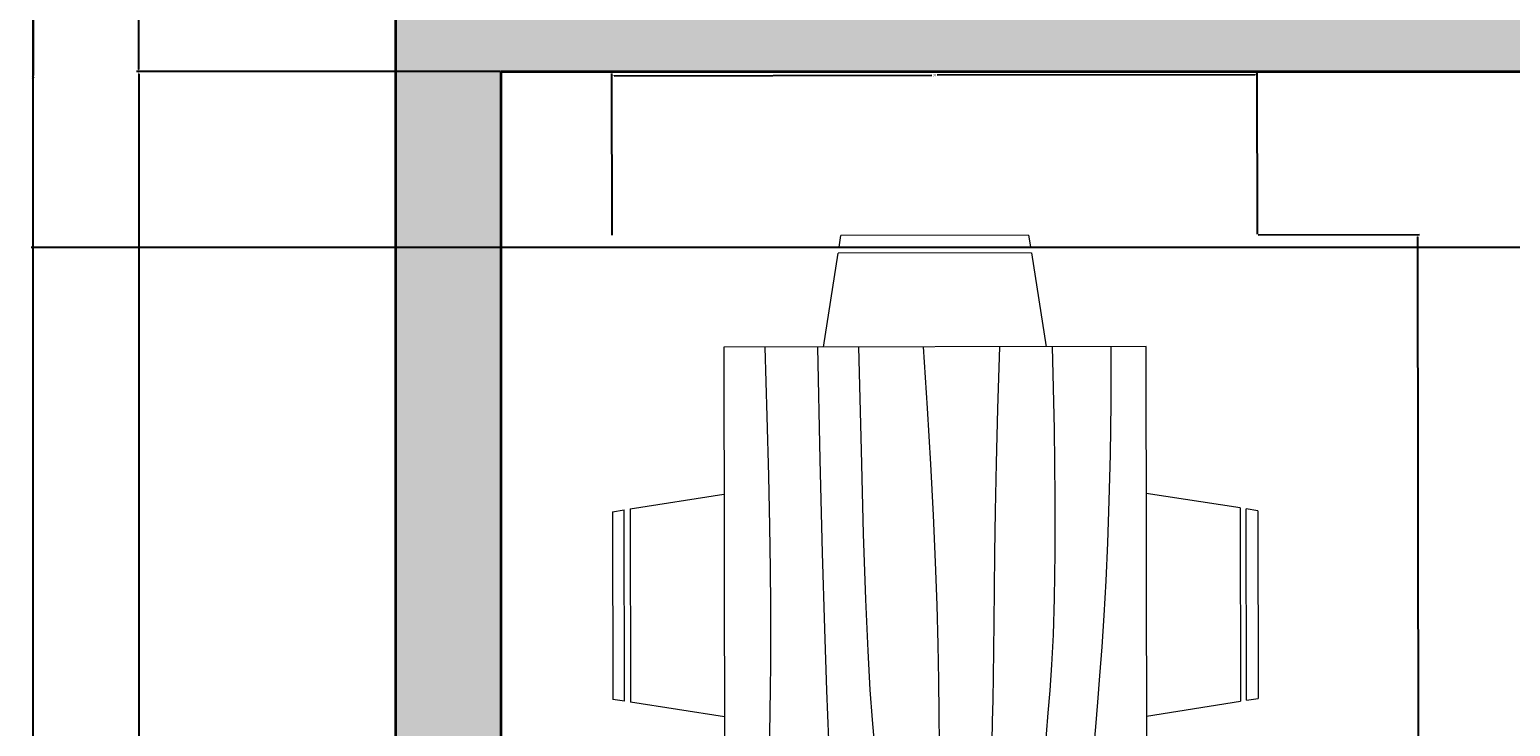
# Model space of a CAD drawing. Units: inches. Extents: x -30 to 437, y -29 to 647.
# Tile 2 of 15: x -30 to 97, y 113 to 172. Entities that reach past the tile are written whole.
import ezdxf

# ---------------------------------------------------------------- set-up
doc = ezdxf.new("R2010")
doc.units = ezdxf.units.IN
doc.header["$MEASUREMENT"] = 0
for name, color, linetype, lineweight in [('A-ANNO-DIMS', 2, 'Continuous', 18), ('A-WALL', 7, 'Continuous', 35), ('furniture', 220, 'Continuous', 18)]:
    doc.layers.add(name, color=color, linetype=linetype, lineweight=lineweight)
doc.layers.add('A-WALL-PATT', color=251, linetype='Continuous', lineweight=13, true_color=0x636466)
doc.styles.get("Standard").update_dxf_attribs({"font": 'arial.ttf'})
doc.dimstyles.get("Standard").update_dxf_attribs({"dimtxt": 0.18, "dimasz": 0.18, "dimexe": 0.18, "dimexo": 0.0625, "dimgap": 0.09, "dimtad": 0, "dimtih": 1, "dimtoh": 1, "dimdec": 4, "dimzin": 0, "dimdsep": 46, "dimtxsty": 'Standard', "dimcen": 0.09, "dimadec": 0, "dimazin": 0, "dimtfac": 1, "dimtdec": 4, "dimtofl": 0, "dimtmove": 0, "dimatfit": 3, "dimfxl": 1, "dimtolj": 1, "dimtzin": 0, "dimarcsym": 0})

# ---------------------------------------------------------------- blocks, each defined once
blk = doc.blocks.new('Dining Set - 36 x 72 in.')
for p, q in [((-22, 27.5), (-22.1562, 26.50042)), ((-22, 27.5), (-6, 27.5)), ((-5.8437, 26.49966), (-6, 27.5)), ((6, 27.5), (5.8438, 26.50042)), ((6, 27.5), (22, 27.5)), ((22.1563, 26.49966), (22, 27.5)), ((-22.2343, 26.00059), (-23.4847, 17.99762)), ((-22.2304, 26), (-5.7608, 26)), ((-5.8416, 26.5), (-22.1534, 26.5)), ((-4.5152, 17.99762), (-5.7655, 25.99926)), ((5.7657, 26.00059), (4.5153, 17.99762)), ((5.7696, 26), (22.2392, 26)), ((22.1584, 26.5), (5.8466, 26.5)), ((23.4848, 17.99762), (22.2345, 25.99926)), ((36, 18), (-36, 18)), ((-36, 18), (-36, -18)), ((36, -18), (36, 18)), ((-44.0006, 8.23428), (-35.9976, 9.48474)), ((44.0006, 8.23428), (35.9976, 9.48474)), ((-45.5, 8), (-44.5004, 8.15617)), ((-45.5, 8), (-45.5, -8)), ((-44.5, -8.15843), (-44.5, 8.15338)), ((-44, 8.23041), (-44, -8.23915)), ((44, 8.23041), (44, -8.23915)), ((44.5, -8.15843), (44.5, 8.15338)), ((45.5, 8), (44.5005, 8.15617)), ((45.5, 8), (45.5, -8)), ((-44.4997, -8.15631), (-45.5, -8)), ((-35.9976, -9.48476), (-43.9993, -8.2345)), ((35.9976, -9.48476), (43.9993, -8.2345)), ((44.4997, -8.15631), (45.5, -8)), ((-36, -18), (36, -18)), ((-22.2343, -26.0006), (-23.4847, -17.99762)), ((-4.5152, -17.99762), (-5.7655, -25.99928)), ((5.7657, -26.0006), (4.5153, -17.99762)), ((23.4848, -17.99762), (22.2345, -25.99928)), ((-22.2304, -26), (-5.7608, -26)), ((-22, -27.5), (-22.1562, -26.50044)), ((-5.8416, -26.5), (-22.1534, -26.5)), ((-5.8437, -26.49967), (-6, -27.5)), ((5.7696, -26), (22.2392, -26)), ((6, -27.5), (5.8438, -26.50044)), ((22.1584, -26.5), (5.8466, -26.5)), ((22.1563, -26.49967), (22, -27.5)), ((-22, -27.5), (-6, -27.5)), ((6, -27.5), (22, -27.5))]:
    blk.add_line(p, q)
for points in [[(-36, 15), (-31.1772, 14.97754), (-26.8079, 14.91406), (-22.8538, 14.81543), (-19.276, 14.6875), (-16.0362, 14.53613), (-13.0957, 14.36718), (-10.4159, 14.18652), (-7.9583, 14), (-5.6904, 13.81315), (-3.6035, 13.63021), (-1.6954, 13.45508), (0.0365, 13.29166), (1.5945, 13.14388), (2.9811, 13.01562), (4.1988, 12.9108), (5.25, 12.83333), (6.1393, 12.78613), (6.8802, 12.76823), (7.4883, 12.77767), (7.9792, 12.8125), (8.3685, 12.87077), (8.6719, 12.95052), (8.9049, 13.0498), (9.0833, 13.16666), (9.2205, 13.29899), (9.3216, 13.44401), (9.3895, 13.59879), (9.4271, 13.76041), (9.4373, 13.92594), (9.4232, 14.09245), (9.3875, 14.257), (9.3333, 14.41666), (9.2638, 14.56917), (9.1836, 14.71484), (9.0975, 14.85465), (9.0104, 14.98958), (8.9272, 15.1206), (8.8529, 15.2487), (8.7922, 15.37483), (8.75, 15.5), (8.7305, 15.62467), (8.7344, 15.74739), (8.7617, 15.86621), (8.8125, 15.97916), (8.8867, 16.08431), (8.9844, 16.17968), (9.1055, 16.26334), (9.25, 16.33333), (9.4189, 16.38802), (9.6172, 16.42708), (9.8506, 16.45052), (10.125, 16.45833), (10.4463, 16.45052), (10.8203, 16.42708), (11.2529, 16.38802), (11.75, 16.33333), (12.3184, 16.26318), (12.9694, 16.17838), (13.7151, 16.07991), (14.5677, 15.96875), (15.5395, 15.84586), (16.6426, 15.71224), (17.8893, 15.56884), (19.2917, 15.41666), (20.859, 15.25667), (22.5879, 15.08984), (24.4721, 14.91715), (26.5052, 14.73958), (28.6809, 14.5581), (30.9929, 14.3737), (33.4347, 14.18733), (36, 14)], [(-36, 10), (-28.9766, 10.14274), (-23.1725, 10.20442), (-18.4241, 10.19775), (-14.5677, 10.13541), (-11.4399, 10.03011), (-8.877, 9.89453), (-6.7154, 9.74137), (-4.7917, 9.58333), (-2.9698, 9.43082), (-1.2246, 9.28515), (0.4415, 9.14534), (2.026, 9.01041), (3.5266, 8.87939), (4.9408, 8.7513), (6.266, 8.62516), (7.5, 8.5), (8.6411, 8.37549), (9.6914, 8.2539), (10.6538, 8.13818), (11.5312, 8.03125), (12.3267, 7.93603), (13.043, 7.85547), (13.6831, 7.79248), (14.25, 7.75), (14.7471, 7.7303), (15.1797, 7.73307), (15.5537, 7.75732), (15.875, 7.80208), (16.1494, 7.86637), (16.3828, 7.94922), (16.5811, 8.04964), (16.75, 8.16666), (16.8944, 8.29915), (17.0143, 8.44531), (17.1089, 8.60319), (17.1771, 8.77083), (17.218, 8.94629), (17.2305, 9.1276), (17.2137, 9.31282), (17.1667, 9.5), (17.0895, 9.6875), (16.987, 9.875), (16.8649, 10.0625), (16.7292, 10.25), (16.5856, 10.4375), (16.4401, 10.625), (16.2985, 10.8125), (16.1667, 11), (16.05, 11.18733), (15.9518, 11.3737), (15.8752, 11.5581), (15.8229, 11.73958), (15.798, 11.91715), (15.8034, 12.08984), (15.842, 12.25667), (15.9167, 12.41666), (16.0295, 12.56836), (16.1784, 12.70833), (16.3605, 12.83268), (16.5729, 12.9375), (16.8127, 13.01888), (17.0768, 13.07291), (17.3625, 13.0957), (17.6667, 13.08333), (17.9894, 13.03312), (18.3418, 12.94726), (18.7382, 12.82918), (19.1927, 12.68229), (19.7195, 12.51001), (20.3327, 12.31575), (21.0465, 12.10294), (21.875, 11.875), (22.8357, 11.63354), (23.959, 11.37304), (25.2786, 11.08618), (26.8282, 10.76562), (28.6414, 10.40405), (30.752, 9.99414), (33.1936, 9.52856), (36, 9)], [(-36, 5.5), (-30.7157, 5.3348), (-26.069, 5.20963), (-21.9946, 5.11767), (-18.4271, 5.05208), (-15.3009, 5.00602), (-12.5508, 4.97265), (-10.1112, 4.94515), (-7.9167, 4.91666), (-5.909, 4.88167), (-4.0586, 4.83984), (-2.3429, 4.79215), (-0.7396, 4.73958), (0.7739, 4.6831), (2.22, 4.6237), (3.6213, 4.56233), (5, 4.5), (6.373, 4.43782), (7.7344, 4.3776), (9.0723, 4.32129), (10.375, 4.27083), (11.6309, 4.22819), (12.8281, 4.19531), (13.9551, 4.17415), (15, 4.16666), (15.954, 4.17448), (16.819, 4.19791), (17.6001, 4.23698), (18.3021, 4.29166), (18.9299, 4.36198), (19.4883, 4.44791), (19.9823, 4.54948), (20.4167, 4.66666), (20.7969, 4.79899), (21.1302, 4.94401), (21.4245, 5.09879), (21.6875, 5.26041), (21.9271, 5.42594), (22.1511, 5.59245), (22.3672, 5.757), (22.5834, 5.91666), (22.8065, 6.06868), (23.0404, 6.21093), (23.2879, 6.34147), (23.5521, 6.45833), (23.8358, 6.55957), (24.142, 6.64323), (24.4735, 6.70735), (24.8334, 6.75), (25.2235, 6.76969), (25.642, 6.76692), (26.0858, 6.74267), (26.5521, 6.69791), (27.0379, 6.63362), (27.5404, 6.55078), (28.0565, 6.45036), (28.5834, 6.33333), (29.1242, 6.19987), (29.7071, 6.04687), (30.3661, 5.87044), (31.1354, 5.66666), (32.0493, 5.43164), (33.142, 5.16146), (34.4475, 4.85221), (36, 4.5)], [(-36, -1), (-30.7915, -0.6591), (-26.0195, -0.38216), (-21.6519, -0.16284), (-17.6563, 0.00521), (-14.0005, 0.12833), (-10.6523, 0.21289), (-7.5796, 0.26522), (-4.75, 0.29166), (-2.134, 0.29793), (0.2878, 0.28711), (2.5317, 0.26163), (4.6146, 0.22396), (6.5529, 0.17651), (8.3633, 0.12174), (10.0623, 0.06209), (11.6667, 0), (13.1899, -0.06201), (14.6341, -0.1211), (15.9982, -0.17432), (17.2813, -0.21875), (18.4823, -0.25147), (19.6003, -0.26953), (20.6343, -0.27002), (21.5834, -0.25), (22.4481, -0.20768), (23.2357, -0.14584), (23.9549, -0.06836), (24.6146, 0.02083), (25.2235, 0.11784), (25.7904, 0.21875), (26.3241, 0.31966), (26.8334, 0.41666), (27.3265, 0.50618), (27.8099, 0.58593), (28.2894, 0.65397), (28.7709, 0.70833), (29.2601, 0.74707), (29.763, 0.76823), (30.2855, 0.76985), (30.8334, 0.75), (31.4088, 0.70784), (31.9994, 0.64713), (32.589, 0.57275), (33.1615, 0.48958), (33.7008, 0.4025), (34.1908, 0.3164), (34.6153, 0.23616), (34.9584, 0.16666), (35.2099, 0.11165), (35.3848, 0.07031), (35.504, 0.04069), (35.5886, 0.02083), (35.6594, 0.00879), (35.7377, 0.0026), (35.8442, 0.00032), (36, 0)], [(-36, -6.5), (-27.1843, -6.31267), (-20.084, -6.1263), (-14.469, -5.9419), (-10.1094, -5.76042), (-6.7752, -5.58285), (-4.2363, -5.41016), (-2.2629, -5.24333), (-0.625, -5.08334), (0.8708, -4.93099), (2.2715, -4.78646), (3.5872, -4.64974), (4.8281, -4.52084), (6.0046, -4.39974), (7.127, -4.28646), (8.2053, -4.18099), (9.25, -4.08334), (10.2705, -3.99382), (11.2734, -3.91407), (12.2647, -3.84603), (13.25, -3.79167), (14.2354, -3.75293), (15.2266, -3.73177), (16.2295, -3.73015), (17.25, -3.75), (18.2912, -3.79248), (19.3451, -3.85547), (20.4009, -3.93604), (21.4479, -4.03125), (22.4754, -4.13819), (23.4727, -4.25391), (24.4289, -4.37549), (25.3334, -4.5), (26.1785, -4.62492), (26.9694, -4.74935), (27.7145, -4.87281), (28.4219, -4.99479), (29.1, -5.11483), (29.7572, -5.23242), (30.4016, -5.34709), (31.0417, -5.45834), (31.6837, -5.56437), (32.3262, -5.65821), (32.9658, -5.73153), (33.599, -5.77604), (34.2224, -5.78345), (34.8327, -5.74545), (35.4264, -5.65373), (36, -5.5)], [(-36, -10), (-26.4022, -9.81299), (-18.4675, -9.62891), (-11.9839, -9.45069), (-6.7396, -9.28125), (-2.5226, -9.12354), (0.8789, -8.98047), (3.6769, -8.85498), (6.0833, -8.75), (8.2767, -8.66765), (10.3021, -8.60677), (12.1712, -8.56543), (13.8958, -8.54167), (15.4876, -8.53353), (16.9583, -8.53907), (18.3197, -8.55632), (19.5834, -8.58334), (20.7616, -8.61841), (21.8685, -8.66081), (22.9188, -8.71004), (23.9271, -8.76563), (24.9081, -8.82707), (25.8763, -8.89388), (26.8465, -8.96558), (27.8334, -9.04167), (28.8474, -9.12118), (29.8828, -9.20117), (30.93, -9.27824), (31.9792, -9.34896), (33.0205, -9.40991), (34.0443, -9.45768), (35.0407, -9.48885), (36, -9.5)], [(-36, -14.5), (-30.0881, -14.33513), (-25.0332, -14.21224), (-20.7312, -14.12647), (-17.0781, -14.07292), (-13.97, -14.04671), (-11.3027, -14.04297), (-8.9724, -14.05681), (-6.875, -14.08334), (-4.9224, -14.11833), (-3.0905, -14.16016), (-1.3709, -14.20785), (0.2448, -14.26042), (1.7647, -14.3169), (3.1973, -14.3763), (4.5507, -14.43767), (5.8333, -14.5), (7.0554, -14.5621), (8.235, -14.62175), (9.3922, -14.67652), (10.5469, -14.72396), (11.7192, -14.76164), (12.929, -14.78711), (14.1965, -14.79794), (15.5417, -14.79167), (16.9933, -14.76424), (18.6152, -14.70508), (20.4804, -14.60197), (22.6615, -14.44271), (25.2312, -14.21509), (28.2624, -13.9069), (31.8277, -13.50594), (36, -13)]]:
    blk.add_lwpolyline(points)
blk = doc.blocks.new('*D19')
at = {"layer": 'A-ANNO-DIMS', "color": 0, "lineweight": -2, "transparency": 16777216}
for p, q in [((75.18, 154.64), (88.95, 154.66)), ((88.77, 154.48), (88.84, 109.34)), ((88.91, 63.84), (88.84, 108.98)), ((75.32, 63.64), (89.09, 63.66))]:
    blk.add_line(p, q, dxfattribs=at)
at = {"layer": 'A-ANNO-DIMS', "color": 0, "transparency": 16777216}
for points in [[(88.8, 154.48), (88.74, 154.48), (88.77, 154.66)], [(88.94, 63.84), (88.88, 63.84), (88.91, 63.66)]]:
    blk.add_solid(points, dxfattribs=at)
at = {"layer": 'Defpoints', "color": 0, "transparency": 16777216}
for p in [(75.12, 154.64), (75.26, 63.64), (88.91, 63.66)]:
    blk.add_point(p, dxfattribs=at)
at = {"layer": 'A-ANNO-DIMS', "color": 0, "transparency": 16777216, "insert": (88.84, 109.16), "char_height": 0.18, "attachment_point": 5}
blk.add_mtext('\\A1;DINING SET 91', dxfattribs=at)
blk = doc.blocks.new('*D20')
at = {"layer": 'A-ANNO-DIMS', "color": 0, "lineweight": -2, "transparency": 16777216}
for p, q in [((20.12, 154.62), (20.1, 168.38)), ((20.28, 168.2), (47.38, 168.25)), ((74.92, 168.29), (47.82, 168.25)), ((75.12, 154.7), (75.1, 168.47))]:
    blk.add_line(p, q, dxfattribs=at)
at = {"layer": 'A-ANNO-DIMS', "color": 0, "transparency": 16777216}
for points in [[(20.28, 168.23), (20.28, 168.17), (20.1, 168.2)], [(74.92, 168.32), (74.92, 168.26), (75.1, 168.29)]]:
    blk.add_solid(points, dxfattribs=at)
at = {"layer": 'Defpoints', "color": 0, "transparency": 16777216}
for p in [(75.1, 168.29), (20.12, 154.55), (75.12, 154.64)]:
    blk.add_point(p, dxfattribs=at)
at = {"layer": 'A-ANNO-DIMS', "color": 0, "transparency": 16777216, "insert": (47.6, 168.25), "char_height": 0.18, "attachment_point": 5}
blk.add_mtext('\\A1;55', dxfattribs=at)
blk = doc.blocks.new('*D26')
at = {"layer": 'A-ANNO-DIMS', "color": 0, "lineweight": -2, "transparency": 16777216}
for p, q in [((1.61, 615.55), (-29.41, 615.55)), ((-29.23, 615.37), (-29.23, 308.98)), ((-29.23, 2.23), (-29.23, 308.62)), ((1.61, 2.05), (-29.41, 2.05))]:
    blk.add_line(p, q, dxfattribs=at)
at = {"layer": 'A-ANNO-DIMS', "color": 0, "transparency": 16777216}
for points in [[(-29.26, 615.37), (-29.2, 615.37), (-29.23, 615.55)], [(-29.26, 2.23), (-29.2, 2.23), (-29.23, 2.05)]]:
    blk.add_solid(points, dxfattribs=at)
at = {"layer": 'Defpoints', "color": 0, "transparency": 16777216}
for p in [(-29.23, 615.55), (1.67, 615.55), (1.67, 2.05)]:
    blk.add_point(p, dxfattribs=at)
at = {"layer": 'A-ANNO-DIMS', "color": 0, "transparency": 16777216, "insert": (-29.23, 308.8), "char_height": 0.18, "attachment_point": 5}
blk.add_mtext('\\A1;613.5', dxfattribs=at)
blk = doc.blocks.new('*D30')
at = {"layer": 'A-ANNO-DIMS', "color": 0, "lineweight": -2, "transparency": 16777216}
for p, q in [((10.61, 168.55), (-20.41, 168.55)), ((-20.23, 168.37), (-20.23, 89.98)), ((-20.23, 11.23), (-20.23, 89.62)), ((10.61, 11.05), (-20.41, 11.05))]:
    blk.add_line(p, q, dxfattribs=at)
at = {"layer": 'A-ANNO-DIMS', "color": 0, "transparency": 16777216}
for points in [[(-20.26, 168.37), (-20.2, 168.37), (-20.23, 168.55)], [(-20.26, 11.23), (-20.2, 11.23), (-20.23, 11.05)]]:
    blk.add_solid(points, dxfattribs=at)
at = {"layer": 'Defpoints', "color": 0, "transparency": 16777216}
for p in [(-20.23, 168.55), (10.67, 168.55), (10.67, 11.05)]:
    blk.add_point(p, dxfattribs=at)
at = {"layer": 'A-ANNO-DIMS', "color": 0, "transparency": 16777216, "insert": (-20.23, 89.8), "char_height": 0.18, "attachment_point": 5}
blk.add_mtext('\\A1;157.5', dxfattribs=at)
blk = doc.blocks.new('*D31')
at = {"layer": 'A-ANNO-DIMS', "color": 0, "lineweight": -2, "transparency": 16777216}
for p, q in [((10.61, 233.55), (-20.41, 233.55)), ((-20.23, 233.37), (-20.23, 201.23)), ((-20.23, 168.73), (-20.23, 200.87)), ((10.61, 168.55), (-20.41, 168.55))]:
    blk.add_line(p, q, dxfattribs=at)
at = {"layer": 'A-ANNO-DIMS', "color": 0, "transparency": 16777216}
for points in [[(-20.26, 233.37), (-20.2, 233.37), (-20.23, 233.55)], [(-20.26, 168.73), (-20.2, 168.73), (-20.23, 168.55)]]:
    blk.add_solid(points, dxfattribs=at)
at = {"layer": 'Defpoints', "color": 0, "transparency": 16777216}
for p in [(-20.23, 233.55), (10.67, 233.55), (10.67, 168.55)]:
    blk.add_point(p, dxfattribs=at)
at = {"layer": 'A-ANNO-DIMS', "color": 0, "transparency": 16777216, "insert": (-20.23, 201.05), "char_height": 0.18, "attachment_point": 5}
blk.add_mtext('\\A1;65', dxfattribs=at)
blk = doc.blocks.new('*D52')
at = {"layer": 'A-ANNO-DIMS', "color": 0, "lineweight": -2, "transparency": 16777216}
for p, q in [((367.61, 182.55), (-29.41, 182.55)), ((-29.23, 182.37), (-29.23, 168.23)), ((-29.23, 153.73), (-29.23, 167.87)), ((396.61, 153.55), (-29.41, 153.55))]:
    blk.add_line(p, q, dxfattribs=at)
at = {"layer": 'A-ANNO-DIMS', "color": 0, "transparency": 16777216}
for points in [[(-29.26, 182.37), (-29.2, 182.37), (-29.23, 182.55)], [(-29.26, 153.73), (-29.2, 153.73), (-29.23, 153.55)]]:
    blk.add_solid(points, dxfattribs=at)
at = {"layer": 'Defpoints', "color": 0, "transparency": 16777216}
for p in [(367.67, 182.55), (-29.23, 153.55), (396.67, 153.55)]:
    blk.add_point(p, dxfattribs=at)
at = {"layer": 'A-ANNO-DIMS', "color": 0, "transparency": 16777216, "insert": (-29.23, 168.05), "char_height": 0.18, "attachment_point": 5}
blk.add_mtext('\\A1;29', dxfattribs=at)

msp = doc.modelspace()

# ---------------------------------------------------------------- hatches: boundary and pattern name
at = {"layer": 'A-WALL-PATT'}
h = msp.add_hatch(color=256, dxfattribs=at)
h.dxf.hatch_style = 1
h.paths.add_polyline_path([(393.6054, 183.2352), (369.6054, 183.2352), (369.6054, 213.2352), (393.6054, 213.2352), (393.6054, 207.2352), (394.6054, 207.2352), (394.6054, 211.2352), (395.6054, 211.2352), (395.6054, 185.2352), (394.6054, 185.2352), (394.6054, 189.2352), (393.6054, 189.2352)], flags=0)
h.paths.add_polyline_path([(384.6054, 189.2352, -1), (390.6054, 189.2352, -1)], flags=0)
h.paths.add_polyline_path([(385.6054, 189.2352, -1), (389.6054, 189.2352, -1)], flags=0)
h.paths.add_polyline_path([(374.6054, 189.2352, -1), (382.6054, 189.2352, -1)], flags=0)
h.paths.add_polyline_path([(386.6054, 189.2352, -1), (388.6054, 189.2352, -1)], flags=0)
h.paths.add_polyline_path([(375.6054, 189.2352, -1), (381.6054, 189.2352, -1)], flags=0)
h.paths.add_polyline_path([(376.6054, 189.2352, -1), (380.6054, 189.2352, -1)], flags=0)
h.paths.add_polyline_path([(377.6054, 189.2352, -1), (379.6054, 189.2352, -1)], flags=0)
h.paths.add_polyline_path([(390.6054, 195.2352), (374.6054, 195.2352), (374.6054, 201.2352), (390.6054, 201.2352)], flags=0)
h.paths.add_polyline_path([(389.6054, 196.2352), (375.6054, 196.2352), (375.6054, 200.2352), (389.6054, 200.2352)], flags=0)
h.paths.add_polyline_path([(383.6054, 207.2352, -1), (391.6054, 207.2352, -1)], flags=0)
h.paths.add_polyline_path([(384.6054, 207.2352, -1), (390.6054, 207.2352, -1)], flags=0)
h.paths.add_polyline_path([(385.6054, 207.2352, -1), (389.6054, 207.2352, -1)], flags=0)
h.paths.add_polyline_path([(386.6054, 207.2352, -1), (388.6054, 207.2352, -1)], flags=0)
h.paths.add_polyline_path([(375.6054, 207.2352, -1), (381.6054, 207.2352, -1)], flags=0)
h.paths.add_polyline_path([(376.6054, 207.2352, -1), (380.6054, 207.2352, -1)], flags=0)
h.paths.add_polyline_path([(377.6054, 207.2352, -1), (379.6054, 207.2352, -1)], flags=0)
h.paths.add_polyline_path([(305.5437, 160.3663, -0.41421356), (304.0437, 158.8663), (271.0437, 158.8663, -0.41421356), (269.5437, 160.3663), (269.5437, 178.3663, -0.41421356), (271.0437, 179.8663), (304.0437, 179.8663, -0.41421356), (305.5437, 178.3663)], flags=0)
h.paths.add_polyline_path([(304.0437, 165.3663, -0.41421356), (303.0437, 164.3663), (289.2937, 164.3663, -0.41421356), (288.2937, 165.3663), (288.2937, 177.3663, -0.41421356), (289.2937, 178.3663), (303.0437, 178.3663, -0.41421356), (304.0437, 177.3663)], flags=0)
h.paths.add_polyline_path([(296.5437, 171.3663, -1), (295.5437, 171.3663, -1)], flags=0)
h.paths.add_polyline_path([(286.7937, 165.3663, -0.41421356), (285.7937, 164.3663), (272.0437, 164.3663, -0.41421356), (271.0437, 165.3663), (271.0437, 177.3663, -0.41421356), (272.0437, 178.3663), (285.7937, 178.3663, -0.41421356), (286.7937, 177.3663)], flags=0)
h.paths.add_polyline_path([(279.5437, 171.3663, -1), (278.5437, 171.3663, -1)], flags=0)
h.paths.add_polyline_path([(360.6737, 290.5474), (360.6737, 300.5474), (396.6737, 300.5474), (396.6737, 290.5474)], flags=0)
h.paths.add_polyline_path([(259.6737, 124.5474), (259.6737, 114.5474), (171.6737, 114.5474), (171.6737, 124.5474)], flags=0)
h.paths.add_polyline_path([(288.0737, 215.3705), (286.7097, 214.583), (268.7097, 245.7599), (270.0737, 246.5474)], flags=0)
h.paths.add_polyline_path([(259.6737, 168.5474), (256.6737, 168.5474), (256.6737, 173.5474), (256.6737, 179.0224), (255.8753, 177.6395), (224.2956, 195.872, 0.12053744), (220.1737, 179.0224, 0.12053744), (216.0518, 195.872), (184.4721, 177.6395), (183.6737, 179.0224), (215.2836, 197.2724), (216.0821, 195.8895), (216.0518, 195.872, -0.12053744), (220.1737, 179.0224, -0.12053744), (224.2956, 195.872), (224.2653, 195.8895), (225.0638, 197.2724), (256.6737, 179.0224), (256.6737, 173.5474), (259.6737, 173.5474)], flags=0)
h.paths.add_polyline_path([(386.7943, 325.4601), (372.6871, 325.4601), (372.6871, 339.5673), (386.7943, 339.5673)], flags=0)
h.paths.add_polyline_path([(359.5875, 343.7429), (357.7905, 343.7429), (357.7905, 327.9179), (359.3933, 327.9179, 0.41420885), (361.5302, 330.0549), (361.5302, 341.8434, 0.41436161)], flags=0)
h.paths.add_polyline_path([(341.7887, 323.1235, -0.11921667), (340.7839, 323.1235)], flags=0)
h.paths.add_polyline_path([(379.6332, 328.8632), (379.6332, 332.2699), (376.0992, 332.2699, 0.39427733)], flags=0)
h.paths.add_polyline_path([(375.5299, 332.459, -1), (383.8511, 332.459, -1)], flags=0)
h.paths.add_polyline_path([(388.9363, 344.7425), (372.5309, 344.7425, -0.41421356), (370.394, 346.8794), (370.394, 347.5594, -0.39085173), (372.3472, 349.7005, -0.43951011), (370.394, 351.4933), (370.394, 365.1894, -0.40305452), (372.2191, 367.1298, -0.41839453), (370.394, 368.9291), (370.394, 382.6251, -0.40885826), (372.2519, 384.5722, -0.42377324), (370.394, 386.3707), (370.394, 400.0667, -0.38660687), (372.1327, 402.0094), (372.531, 402.0094, -0.41421834), (370.394, 404.1464), (370.394, 404.7778, -0.41420891), (372.5309, 406.9147), (388.9363, 406.9147, -0.41421821), (391.0733, 404.7778), (391.0733, 346.8794, -0.41421356)], flags=0)
edge = h.paths.add_edge_path(flags=0)
edge.add_spline(control_points=[(349.3585, 363.204), (349.0859, 363.204), (348.8133, 363.2227), (348.2712, 363.2973), (348.0016, 363.3531), (347.3533, 363.5328), (346.9776, 363.6755), (346.2445, 364.0308), (345.887, 364.2432), (345.1953, 364.7329), (344.8611, 365.0101), (344.2197, 365.6237), (343.9125, 365.9603), (343.211, 366.8336), (342.8313, 367.3965), (342.1401, 368.6117), (341.8286, 369.2641), (341.2807, 370.64), (341.0443, 371.3636), (340.6522, 372.8619), (340.4964, 373.6367), (340.2695, 375.2158), (340.1983, 376.0203), (340.142, 377.6365), (340.157, 378.4483), (340.2729, 380.0567), (340.3738, 380.8533), (340.6589, 382.4093), (340.8432, 383.1686), (341.2906, 384.629), (341.5538, 385.3301), (342.1531, 386.6544), (342.4891, 387.2776), (343.2266, 388.4288), (343.6281, 388.9567), (344.4879, 389.9012), (344.9463, 390.3178), (345.7981, 390.9428), (346.182, 391.1771), (346.9712, 391.5648), (347.3766, 391.7182), (348.2004, 391.9387), (348.6189, 392.0058), (349.4588, 392.0508), (349.8801, 392.0288), (350.7146, 391.8966), (351.1278, 391.7865), (351.9366, 391.4822), (352.3323, 391.2882), (353.0989, 390.8223), (353.4699, 390.5504), (354.1819, 389.9355), (354.5229, 389.5924), (355.1706, 388.8418), (355.4772, 388.4343), (356.1315, 387.4422), (356.4671, 386.8397), (357.0692, 385.5581), (357.3356, 384.879), (357.7933, 383.4624), (357.9846, 382.725), (358.2875, 381.2112), (358.3992, 380.4349), (358.5404, 378.8643), (358.5699, 378.0699), (358.546, 376.4841), (358.4926, 375.6928), (358.3042, 374.1343), (358.1692, 373.3672), (357.8207, 371.8774), (357.6072, 371.1549), (357.1067, 369.7735), (356.8196, 369.1148), (356.1782, 367.8787), (355.8238, 367.3013), (355.0551, 366.244), (354.6408, 365.7641), (353.7607, 364.9161), (353.2948, 364.5481), (352.445, 364.0149), (352.0701, 363.822), (351.3034, 363.5117), (350.9116, 363.3943), (350.1325, 363.2418), (349.7455, 363.204), (349.3585, 363.204)], knot_values=[3.14159265, 3.14159265, 3.14159265, 3.14159265, 3.22691715, 3.22691715, 3.31224165, 3.31224165, 3.43426671, 3.43426671, 3.55629177, 3.55629177, 3.67831683, 3.67831683, 3.8003419, 3.8003419, 3.97157384, 3.97157384, 4.14280577, 4.14280577, 4.31403771, 4.31403771, 4.48526965, 4.48526965, 4.65650159, 4.65650159, 4.82773353, 4.82773353, 4.99896547, 4.99896547, 5.1701974, 5.1701974, 5.34142934, 5.34142934, 5.51266128, 5.51266128, 5.68389322, 5.68389322, 5.85512516, 5.85512516, 5.98669107, 5.98669107, 6.11825699, 6.11825699, 6.24982291, 6.24982291, 6.38138882, 6.38138882, 6.51295474, 6.51295474, 6.64452065, 6.64452065, 6.77608657, 6.77608657, 6.90765249, 6.90765249, 7.0392184, 7.0392184, 7.20701563, 7.20701563, 7.37481286, 7.37481286, 7.54261009, 7.54261009, 7.71040732, 7.71040732, 7.87820455, 7.87820455, 8.04600178, 8.04600178, 8.21379901, 8.21379901, 8.38159624, 8.38159624, 8.54939347, 8.54939347, 8.7171907, 8.7171907, 8.88498794, 8.88498794, 9.05278517, 9.05278517, 9.17820699, 9.17820699, 9.30362881, 9.30362881, 9.42477796, 9.42477796, 9.42477796, 9.42477796], degree=3, periodic=0)
edge.add_line((341.1696, 384.3006), (341.2012, 384.2808))
edge = h.paths.add_edge_path(flags=0)
edge.add_line((344.3353, 388.7801), (344.317, 388.7915))
edge.add_ellipse((349.3585, 377.6204), major_axis=(0, -13.7895), ratio=0.62186025, start_angle=-244.867444, end_angle=-124.769923)
h.paths.add_polyline_path([(163.6737, 163.1474), (132.4968, 145.1474), (131.7093, 146.5114), (162.8862, 164.5114)], flags=0)
h.paths.add_polyline_path([(366.4355, 409.0896, -0.41423669), (364.2985, 406.9525, -0.4913499), (361.5302, 408.8973), (361.5302, 420.6405, 0.41421356), (359.3932, 422.7775), (357.7905, 422.7775), (357.7905, 406.9525), (359.6317, 406.9525, 0.42741026), (361.5332, 408.9757, 0.39869469), (363.6672, 406.9525, 0.51958103), (366.4355, 409.0895)], flags=0)
h.paths.add_polyline_path([(386.7943, 410.9671), (372.6871, 410.9671), (372.6871, 425.0742), (386.7943, 425.0742)], flags=0)
h.paths.add_polyline_path([(379.6332, 414.3701), (379.6332, 417.7768), (376.0992, 417.7768, 0.39427733)], flags=0)
h.paths.add_polyline_path([(375.5299, 417.966, -1), (383.8511, 417.966, -1)], flags=0)
h.paths.add_polyline_path([(150.0377, 351.583), (148.6737, 352.3705), (166.6737, 383.5474), (168.0377, 382.7599)], flags=0)
h.paths.add_polyline_path([(91.6737, 234.1974), (66.559, 219.6974), (65.9246, 220.7962), (91.0393, 235.2962)], flags=0)
h.paths.add_polyline_path([(255.4612, 443.5834), (254.6737, 444.9474), (285.8506, 462.9474), (286.6381, 461.5834)], flags=0)
h.paths.add_polyline_path([(176.2737, 394.5474), (158.2737, 425.7243), (159.6377, 426.5118), (177.6377, 395.3349)], flags=0)
h.paths.add_polyline_path([(243.6737, 439.5474), (243.0393, 438.4486), (217.9246, 452.9486), (218.559, 454.0474)], flags=0)
h.paths.add_polyline_path([(38.1264, 269.8429), (40.2408, 269.8429), (40.2408, 270.3508), (38.1264, 270.3508)], flags=0)
h.paths.add_polyline_path([(75.7157, 289.9439), (40.2408, 289.9439), (38.1264, 289.6524), (40.2408, 289.6524)], flags=0)
h.paths.add_polyline_path([(75.7157, 270.0846), (77.6447, 270.0846), (77.6697, 270.1626), (75.7175, 270.1626)], flags=0)
h.paths.add_polyline_path([(80.5373, 293.3002), (33.0467, 293.3002), (13.5054, 293.3002), (13.5054, 351.9244), (29.7898, 351.9244), (80.5373, 351.9244)], flags=0)
h.paths.add_polyline_path([(46.0261, 212.466, -0.50131678), (27.1651, 207.5106), (21.165, 209.5107), (21.165, 206.5107), (22.665, 206.5107), (22.665, 203.5107), (21.165, 203.5107), (21.165, 203.0107), (13.165, 203.0107), (13.165, 224.0107), (21.165, 224.0107), (21.165, 217.5107), (27.1649, 219.5106, -0.50132349), (46.0261, 214.5554, -0.13289091)], flags=0)
h.paths.add_polyline_path([(44.688, 211.8666, -0.48007965), (27.165, 209.5107), (27.165, 217.5107, -0.4800795), (44.688, 215.1547, -0.21500378)], flags=0)
h.paths.add_polyline_path([(19.415, 204.0107), (15.165, 204.0107, -0.41421356), (14.165, 204.7607), (14.165, 222.0107, -0.41421356), (14.915, 223.0107), (19.165, 223.0107, -0.41421356), (20.165, 222.2607), (20.165, 205.0107, -0.41421356)], flags=0)
h.paths.add_polyline_path([(32.7608, 269.0719), (31.8439, 269.0719), (31.8439, 268.6134), (13.5054, 268.6134), (13.5054, 291.5366), (31.8439, 291.5366), (32.7608, 291.0781), (32.7608, 280.9919, -1), (32.7608, 279.1581)], flags=0)
h.paths.add_polyline_path([(40.2408, 360.1436), (38.1264, 360.1436), (38.1264, 359.6357), (40.2408, 359.6357)], flags=0)
h.paths.add_polyline_path([(75.7157, 355.2807), (40.2408, 355.2807), (38.1264, 355.5722), (40.2408, 355.5722), (40.2408, 355.2807), (75.7157, 355.2807), (75.7157, 375.5982), (40.2408, 375.5982), (38.1264, 375.3817), (40.2408, 375.3817), (40.2408, 375.5982), (75.7157, 375.5982), (77.9733, 375.062), (75.7175, 375.062), (75.7175, 374.554)], flags=0)
h.paths.add_polyline_path([(42.8174, 299.814, 0.13867074), (34.1602, 294.603), (14.8081, 294.603), (14.8081, 350.6216), (29.8539, 350.6216, 0.09822056)], flags=0)
h.paths.add_polyline_path([(15.8636, 276.7781, -0.30640166), (20.3757, 283.4499), (20.3483, 290.6726), (31.4014, 290.7146), (31.4309, 282.9124), (26.8287, 282.895, -0.26006276), (30.241, 276.7781, -1)], flags=0)
h.paths.add_polyline_path([(26.1332, 276.7781), (23.0523, 273.6972), (19.9714, 276.7781), (23.0523, 279.8589), (23.0523, 283.9209), (21.3493, 283.9145), (20.7006, 283.5219), (20.6907, 286.1226), (23.2914, 286.1325), (25.8936, 285.7522), (27.1939, 285.7572), (28.4928, 286.1522), (31.0935, 286.1621), (31.0918, 286.6172), (25.6303, 286.5965), (25.616, 290.3675), (31.0775, 290.3882), (31.0918, 286.6172), (31.1034, 283.5614), (28.5027, 283.5515), (25.9005, 283.9317), (23.0523, 283.9209), (23.0523, 279.8589)], flags=0)
h.paths.add_polyline_path([(24.0793, 276.7781, -1), (22.0253, 276.7781, -1)], flags=0)
h.paths.add_polyline_path([(35.7687, 302.2895, -0.41421356), (35.2283, 301.2726), (22.2164, 297.2909, -0.41421356), (21.1995, 297.8313), (15.7317, 315.6996, -0.41421356), (16.2721, 316.7165), (18.8554, 317.507), (15.3721, 328.8904, -0.41421356), (15.9125, 329.9073), (28.9244, 333.889, -0.41421356), (29.9414, 333.3486), (35.4091, 315.4802, -0.41421356), (34.8687, 314.4633), (32.2854, 313.6728)], flags=0)
h.paths.add_polyline_path([(361.3728, 532.6207), (302.7487, 532.6207), (302.7487, 580.1113), (302.7487, 599.6527), (361.3728, 599.6527), (361.3728, 583.3682)], flags=0)
h.paths.add_polyline_path([(370.1, 575.0316), (370.1, 572.9172), (370.6079, 572.9172), (370.6079, 575.0316)], flags=0)
h.paths.add_polyline_path([(385.0466, 537.4423), (385.0466, 572.9172), (384.8302, 575.0316), (384.8302, 572.9172)], flags=0)
h.paths.add_polyline_path([(384.5104, 535.3262), (384.5104, 537.4406), (384.0025, 537.4406), (364.7291, 537.4423), (364.7291, 572.9172), (365.0206, 575.0316), (365.0206, 572.9172), (364.7291, 572.9172), (364.7291, 537.4423), (384.5884, 537.4423), (384.5884, 535.5133)], flags=0)
h.paths.add_polyline_path([(384.5884, 535.5133), (383.4945, 535.164), (383.4945, 537.4406), (382.9866, 535.3262), (382.9866, 537.4406), (383.4945, 535.3262), (383.4945, 537.4406), (384.5884, 537.4406)], flags=0)
h.paths.add_polyline_path([(23.874, 286.8174), (21.0132, 286.8065), (21.0004, 290.1875), (23.8612, 290.1983)], flags=0)
h.paths.add_polyline_path([(242.9824, 511.1667), (234.9824, 511.1667), (234.9824, 517.6667), (228.9825, 515.6667, -0.50132349), (210.1213, 520.622, -0.13289091), (210.1213, 522.7114, -0.50131678), (228.9823, 527.6667), (234.9824, 525.6667), (234.9824, 528.6667), (233.4824, 528.6667), (233.4824, 531.6667), (234.9824, 531.6667), (234.9824, 532.1667), (242.9824, 532.1667)], flags=0)
h.paths.add_polyline_path([(236.9824, 512.1667, -0.41421356), (235.9824, 512.9167), (235.9824, 530.1667, -0.41421356), (236.7324, 531.1667), (240.9824, 531.1667, -0.41421356), (241.9824, 530.4167), (241.9824, 513.1667, -0.41421356), (241.2324, 512.1667)], flags=0)
h.paths.add_polyline_path([(279.533, 537.4423), (279.533, 535.5133), (279.6111, 535.4884), (279.6111, 537.4406)], flags=0)
h.paths.add_polyline_path([(279.2913, 575.0316), (279.2913, 572.9172), (279.7992, 572.9172), (279.7992, 575.0316)], flags=0)
h.paths.add_polyline_path([(211.4594, 520.0227, -0.21500378), (211.4594, 523.3107, -0.48007965), (228.9824, 525.6667), (228.9824, 517.6667, -0.4800795)], flags=0)
h.paths.add_polyline_path([(32.7627, 354.1465), (31.8457, 354.1465), (31.8457, 353.688), (13.5054, 353.688), (13.5054, 376.6134), (31.8457, 376.6134), (32.7627, 376.1549), (32.7627, 366.0677, -1), (32.7627, 364.2337)], flags=0)
h.paths.add_polyline_path([(15.9446, 365.1507, -1), (30.3234, 365.1507, -1)], flags=0)
h.paths.add_polyline_path([(41.213, 428.467), (43.3274, 428.467), (43.3274, 428.9749), (41.213, 428.9749)], flags=0)
h.paths.add_polyline_path([(78.8022, 448.568), (43.3274, 448.568), (41.213, 448.2765), (43.3274, 448.2765)], flags=0)
h.paths.add_polyline_path([(78.8022, 428.7087), (80.7313, 428.7087), (80.7562, 428.7868), (78.804, 428.7868)], flags=0)
h.paths.add_polyline_path([(26.2152, 365.1507), (23.134, 362.0696), (20.0529, 365.1507), (23.134, 368.2319)], flags=0)
h.paths.add_polyline_path([(24.1611, 365.1507, -1), (22.107, 365.1507, -1)], flags=0)
h.paths.add_polyline_path([(309.2625, 570.3406, 0.13867074), (304.0514, 578.9978), (304.0514, 598.3499), (360.07, 598.3499), (360.07, 583.3041, 0.09822056)], flags=0)
h.paths.add_polyline_path([(246.6737, 552.5474), (129.6737, 552.5474), (129.6737, 606.5474), (246.6737, 606.5474)], flags=16)
h.paths.add_polyline_path([(373.6822, 580.3953), (363.595, 580.3953), (363.595, 581.3123), (363.1365, 581.3123), (363.1365, 599.6527), (386.0619, 599.6527), (386.0619, 581.3123), (385.6034, 580.3953), (375.5162, 580.3953, -1)], flags=0)
h.paths.add_polyline_path([(83.6239, 451.9244), (36.1333, 451.9244), (16.5919, 451.9244), (16.5919, 510.5485), (32.8764, 510.5485), (83.6239, 510.5485)], flags=0)
h.paths.add_polyline_path([(367.4098, 590.024, -1), (381.7886, 590.024, -1)], flags=0)
h.paths.add_polyline_path([(374.5992, 586.9428), (371.518, 590.024), (374.5992, 593.1052), (377.6803, 590.024)], flags=0)
h.paths.add_polyline_path([(373.5721, 590.024, -1), (375.6262, 590.024, -1)], flags=0)
h.paths.add_polyline_path([(324.9287, 577.7489, -0.41421356), (323.9118, 578.2893), (323.1212, 580.8726), (311.7379, 577.3893, -0.41421356), (310.721, 577.9297), (306.7393, 590.9416, -0.41421356), (307.2797, 591.9585), (325.1481, 597.4263, -0.41421356), (326.165, 596.8859), (326.9555, 594.3026), (338.3388, 597.7859, -0.41421356), (339.3557, 597.2455), (343.3374, 584.2336, -0.41421356), (342.797, 583.2167)], flags=0)
h.paths.add_polyline_path([(300.5265, 580.3972), (290.4404, 580.3972, -1), (288.6065, 580.3972), (278.5203, 580.3972), (278.5203, 581.3142), (278.0619, 581.3142), (278.0619, 599.6527), (300.985, 599.6527), (300.985, 581.3142)], flags=0)
h.paths.add_polyline_path([(300.163, 581.7567), (292.3609, 581.7271), (292.3434, 586.3294, -0.75567924), (279.0378, 590.1057, -0.82536731), (292.8983, 592.7823), (300.1211, 592.8097)], flags=0)
h.paths.add_polyline_path([(299.8367, 582.0805), (296.0656, 582.0662), (293.0098, 582.0546), (292.9999, 584.6553), (293.3802, 587.2575), (293.3694, 590.1057), (289.3074, 590.1057), (286.2265, 587.0248), (283.1456, 590.1057), (286.2265, 593.1866), (289.3074, 590.1057), (293.3694, 590.1057), (293.3629, 591.8088), (292.9703, 592.4575), (295.5711, 592.4673), (295.5809, 589.8666), (295.2007, 587.2644), (295.2056, 585.9641), (295.6006, 584.6652), (295.6105, 582.0645), (296.0656, 582.0662), (296.0449, 587.5277), (299.8159, 587.542)], flags=0)
h.paths.add_polyline_path([(285.1995, 590.1057, -1), (287.2535, 590.1057, -1)], flags=0)
h.paths.add_polyline_path([(299.6467, 589.2969), (296.2658, 589.284), (296.255, 592.1448), (299.6359, 592.1576)], flags=0)
h.paths.add_polyline_path([(35.8473, 427.696), (34.9304, 427.696), (34.9304, 427.2376), (16.5919, 427.2376), (16.5919, 450.1607), (34.9304, 450.1607), (35.8473, 449.7022), (35.8473, 439.6161, -1), (35.8473, 437.7822)], flags=0)
h.paths.add_polyline_path([(18.9502, 435.4022, -0.30640166), (23.4623, 442.074), (23.4349, 449.2968), (34.4879, 449.3387), (34.5175, 441.5366), (29.9152, 441.5191, -0.26006276), (33.3275, 435.4022, -1)], flags=0)
h.paths.add_polyline_path([(29.2197, 435.4022), (26.1389, 432.3213), (23.058, 435.4022), (26.1389, 438.4831), (26.1389, 442.5451), (24.4358, 442.5386), (23.7871, 442.1461), (23.7772, 444.7468), (26.378, 444.7566), (28.9801, 444.3764), (30.2805, 444.3813), (31.5794, 444.7764), (34.1801, 444.7862), (34.1784, 445.2413), (28.7169, 445.2206), (28.7026, 448.9917), (34.164, 449.0124), (34.1784, 445.2413), (34.1899, 442.1855), (31.5892, 442.1756), (28.987, 442.5559), (26.1389, 442.5451), (26.1389, 438.4831)], flags=0)
h.paths.add_polyline_path([(27.1658, 435.4022, -1), (25.1119, 435.4022, -1)], flags=0)
h.paths.add_polyline_path([(45.904, 458.4382, 0.13867074), (37.2467, 453.2271), (17.8947, 453.2271), (17.8947, 509.2457), (32.9405, 509.2457, 0.09822056)], flags=0)
h.paths.add_polyline_path([(26.9605, 445.4415), (24.0997, 445.4307), (24.0869, 448.8116), (26.9477, 448.8225)], flags=0)
h.paths.add_polyline_path([(38.3149, 459.8967), (25.3029, 455.915, -0.41421356), (24.286, 456.4554), (18.8183, 474.3238, -0.41421356), (19.3586, 475.3407), (21.942, 476.1312), (18.4587, 487.5145, -0.41421356), (18.999, 488.5314), (32.011, 492.5131, -0.41421356), (33.0279, 491.9727), (38.4957, 474.1044, -0.41421356), (37.9553, 473.0875), (35.3719, 472.297), (38.8553, 460.9136, -0.41421356)], flags=0)
h.paths.add_polyline_path([(43.3274, 518.7678), (41.213, 518.7678), (41.213, 518.2598), (43.3274, 518.2598)], flags=0)
h.paths.add_polyline_path([(78.8022, 513.9049), (43.3274, 513.9049), (41.213, 514.1964), (43.3274, 514.1964), (43.3274, 513.9049), (78.8022, 513.9049), (78.8022, 534.2223), (43.3274, 534.2223), (41.213, 534.0059), (43.3274, 534.0059), (43.3274, 534.2223), (78.8022, 534.2223), (81.0599, 533.6861), (78.804, 533.6861), (78.804, 533.1782)], flags=0)
h.paths.add_polyline_path([(121.6737, 556.8974), (121.0393, 555.7986), (95.9246, 570.2986), (96.559, 571.3974)], flags=0)
h.paths.add_polyline_path([(35.8493, 512.7707), (34.9322, 512.7707), (34.9322, 512.3122), (16.5919, 512.3122), (16.5919, 535.2376), (34.9322, 535.2376), (35.8493, 534.7791), (35.8493, 524.6919, -1), (35.8493, 522.8579)], flags=0)
h.paths.add_polyline_path([(19.0312, 523.7749, -1), (33.41, 523.7749, -1)], flags=0)
h.paths.add_polyline_path([(26.2206, 520.6937), (23.1394, 523.7749), (26.2206, 526.8561), (29.3018, 523.7749)], flags=0)
h.paths.add_polyline_path([(25.1935, 523.7749, -1), (27.2476, 523.7749, -1)], flags=0)
h.paths.add_polyline_path([(28.4381, 586.0173), (22.438, 588.0173), (22.438, 585.0173), (23.938, 585.0173), (23.938, 582.0173), (22.438, 582.0173), (22.438, 581.5173), (14.438, 581.5173), (14.438, 602.5173), (22.438, 602.5173), (22.438, 596.0173), (28.4379, 598.0173, -0.50132349), (47.2992, 593.062, -0.13289091), (47.2992, 590.9726, -0.50131678)], flags=0)
h.paths.add_polyline_path([(28.438, 588.0174), (28.438, 596.0173, -0.4800795), (45.961, 593.6614, -0.21500378), (45.961, 590.3733, -0.48007965)], flags=0)
h.paths.add_polyline_path([(20.688, 582.5173), (16.438, 582.5173, -0.41421356), (15.438, 583.2673), (15.438, 600.5173, -0.41421356), (16.188, 601.5173), (20.438, 601.5173, -0.41421356), (21.438, 600.7673), (21.438, 583.5173, -0.41421356)], flags=0)
h.paths.add_polyline_path([(171.6737, 2.0474), (171.6737, 104.5474), (259.6737, 104.5474), (259.6737, 148.5474), (396.6737, 148.5474), (396.6737, 2.0474), (405.6737, 2.0474), (405.6737, 615.5474), (1.6737, 615.5474), (1.6737, 2.0474)])
h.paths.add_polyline_path([(171.6737, 104.5474), (259.6737, 104.5474), (259.6737, 210.5474), (264.6737, 210.5474), (264.6737, 153.5474), (396.6737, 153.5474), (396.6737, 249.5474), (264.6737, 249.5474), (264.6737, 246.5474), (259.6737, 246.5474), (259.6737, 254.5474), (396.6737, 254.5474), (396.6737, 434.5474), (290.6737, 434.5474), (290.6737, 439.5474), (396.6737, 439.5474), (396.6737, 606.5474), (251.6737, 606.5474), (251.6737, 439.5474), (254.6737, 439.5474), (254.6737, 434.5474), (243.6737, 434.5474), (243.6737, 439.5474), (246.6737, 439.5474), (246.6737, 547.5474), (186.6737, 547.5474), (186.6737, 439.5474), (214.6737, 439.5474), (214.6737, 434.5474), (186.6737, 434.5474), (186.6737, 430.5474), (181.6737, 430.5474), (181.6737, 547.5474), (121.6737, 547.5474), (121.6737, 552.5474), (124.6737, 552.5474), (124.6737, 606.5474), (10.6737, 606.5474), (10.6737, 552.5474), (92.6737, 552.5474), (92.6737, 547.5474), (10.6737, 547.5474), (10.6737, 391.5474), (181.6737, 391.5474), (181.6737, 394.5474), (186.6737, 394.5474), (186.6737, 386.5474), (171.6737, 386.5474), (171.6737, 383.5474), (166.6737, 383.5474), (166.6737, 386.5474), (10.6737, 386.5474), (10.6737, 238.5474), (62.6737, 238.5474), (62.6737, 233.5474), (10.6737, 233.5474), (10.6737, 173.5474), (94.6737, 173.5474), (94.6737, 233.5474), (91.6737, 233.5474), (91.6737, 238.5474), (166.6737, 238.5474), (166.6737, 347.5474), (171.6737, 347.5474), (171.6737, 233.5474), (99.6737, 233.5474), (99.6737, 173.5474), (127.6737, 173.5474), (127.6737, 168.5474), (10.6737, 168.5474), (10.6737, 11.0474), (166.6737, 11.0474), (166.6737, 168.5474), (163.6737, 168.5474), (163.6737, 173.5474), (183.6737, 173.5474), (183.6737, 168.5474), (171.6737, 168.5474)])

# ---------------------------------------------------------------- linework, layer by layer
at = {"layer": 'A-WALL'}
for p, q in [((10.6737, 168.5474), (127.6737, 168.5474)), ((10.6737, 11.0474), (10.6737, 168.5474))]:
    msp.add_line(p, q, dxfattribs=at)
msp.add_lwpolyline([(171.6737, 2.0474), (1.6737, 2.0474), (1.6737, 615.5474), (405.6737, 615.5474), (405.6737, 2.0474), (396.6737, 2.0474)], dxfattribs=at)

# ---------------------------------------------------------------- block references
at = {"layer": 'furniture', "rotation": 270.0891389700014}
msp.add_blockref('Dining Set - 36 x 72 in.', (47.6887, 109.0958), dxfattribs=at)

# ---------------------------------------------------------------- dimensions: what is measured, and where the dimension line sits
at = {"layer": 'A-ANNO-DIMS'}
for base, p1, p2, angle, override, picture, middle in [((-29.2263, 615.5474), (1.6737, 2.0474), (1.6737, 615.5474), 90, {"dimdec": 1, "dimlfac": 1, "dimrnd": 0, "dimzin": 0, "dimdsep": 46, "dimlunit": 2}, '*D26', (-29.2263, 308.7974)), ((-20.2263, 233.5474), (10.6737, 168.5474), (10.6737, 233.5474), 90, {"dimdec": 0, "dimlfac": 1, "dimrnd": 0, "dimzin": 0, "dimdsep": 46, "dimlunit": 2}, '*D31', (-20.2263, 201.0474)), ((-29.2263, 153.5474), (367.6737, 182.5474), (396.6737, 153.5474), 90, {"dimdec": 0, "dimlfac": 1, "dimrnd": 0, "dimzin": 0, "dimdsep": 46, "dimlunit": 2}, '*D52', (-29.2263, 168.0474)), ((-20.2263, 168.5474), (10.6737, 11.0474), (10.6737, 168.5474), 90, {"dimdec": 1, "dimlfac": 1, "dimrnd": 0, "dimzin": 0, "dimdsep": 46, "dimlunit": 2}, '*D30', (-20.2263, 89.7974)), ((75.0966, 168.2885), (20.1179, 154.553), (75.1178, 154.6385), 0.089139, {"dimdec": 0, "dimlfac": 1, "dimrnd": 0, "dimzin": 0, "dimdsep": 46, "dimlunit": 2}, '*D20', (47.5966, 168.2457))]:
    dim = msp.add_linear_dim(base=base, p1=p1, p2=p2, angle=angle, dimstyle='Standard', override=override, dxfattribs=at)
    dim.commit()
    dim.dimension.update_dxf_attribs({"geometry": picture, "text_midpoint": middle})
dim = msp.add_linear_dim(base=(88.9094, 63.6599), p1=(75.1178, 154.6385), p2=(75.2594, 63.6386), angle=270.089139, text='DINING SET <>', dimstyle='Standard', override={"dimdec": 0, "dimlfac": 1, "dimrnd": 0, "dimzin": 0, "dimdsep": 46, "dimlunit": 2}, dxfattribs=at)
dim.commit()
dim.dimension.update_dxf_attribs({"geometry": '*D19', "text_midpoint": (88.8386, 109.1598)})

doc.saveas('drawing.dxf')
